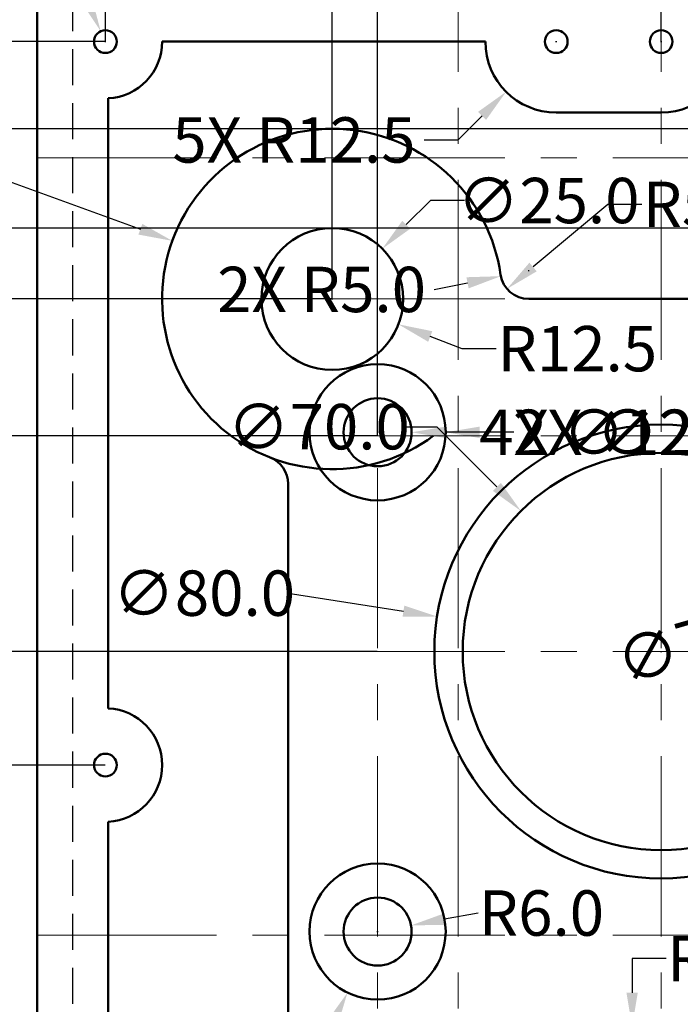
# Model space of a CAD drawing. Units: inches. Extents: x 11765 to 12471, y 10149 to 10793.
# Tile 4 of 8: x 11880 to 11996, y 10530 to 10704. Entities that reach past the tile are written whole.
import ezdxf

# ---------------------------------------------------------------- set-up
doc = ezdxf.new("R2010")
doc.units = ezdxf.units.IN
doc.header["$MEASUREMENT"] = 0
doc.linetypes.add('CENTER', pattern=[50.8, 31.75, -6.35, 6.35, -6.35])
doc.linetypes.add('HIDDEN', pattern=[9.525, 6.35, -3.175])
for name, color, linetype, lineweight in [('M-CNTR', 30, 'CENTER', 18), ('M-DIMS', 2, 'Continuous', 25), ('M-HIDN', 41, 'HIDDEN', 25), ('M-OUTL', 7, 'Continuous', 50)]:
    doc.layers.add(name, color=color, linetype=linetype, lineweight=lineweight)
doc.styles.get("Standard").update_dxf_attribs({"font": 'arial.ttf'})
doc.dimstyles.get("Standard").update_dxf_attribs({"dimtxt": 8, "dimasz": 6, "dimexe": 0.18, "dimexo": 0.0625, "dimgap": 0.09, "dimtad": 0, "dimtoh": 1, "dimdec": 1, "dimzin": 0, "dimdsep": 46, "dimtxsty": 'Standard', "dimcen": 0.09, "dimadec": 0, "dimazin": 0, "dimtfac": 1, "dimtdec": 1, "dimtofl": 0, "dimtmove": 0, "dimatfit": 3, "dimfxl": 1, "dimtolj": 1, "dimtzin": 0, "dimarcsym": 0})

# ---------------------------------------------------------------- blocks, each defined once
blk = doc.blocks.new('*D2')
at = {"layer": 'Defpoints', "color": 0, "transparency": 16777216}
for p in [(11894.91, 10776.05), (11992.91, 10712.15), (11894.91, 10699.65)]:
    blk.add_point(p, dxfattribs=at)
at = {"layer": 'M-DIMS', "color": 0, "lineweight": -2, "transparency": 16777216}
for p, q in [((11894.91, 10699.71), (11894.91, 10776.23)), ((11900.91, 10776.05), (11933.45, 10776.05)), ((11986.91, 10776.05), (11954.38, 10776.05)), ((11992.91, 10712.21), (11992.91, 10776.23))]:
    blk.add_line(p, q, dxfattribs=at)
at = {"layer": 'M-DIMS', "color": 0, "transparency": 16777216}
for points in [[(11900.91, 10777.05), (11900.91, 10775.05), (11894.91, 10776.05)], [(11986.91, 10777.05), (11986.91, 10775.05), (11992.91, 10776.05)]]:
    blk.add_solid(points, dxfattribs=at)
at = {"layer": 'M-DIMS', "color": 0, "transparency": 16777216, "insert": (11943.91, 10776.05), "char_height": 8, "attachment_point": 5}
blk.add_mtext('\\A1;98.0', dxfattribs=at)
blk = doc.blocks.new('*D3')
at = {"layer": 'Defpoints', "color": 0, "transparency": 16777216}
for p in [(11992.91, 10763.84), (11992.91, 10699.65), (11934.91, 10654.29)]:
    blk.add_point(p, dxfattribs=at)
at = {"layer": 'M-DIMS', "color": 0, "lineweight": -2, "transparency": 16777216}
for p, q in [((11934.91, 10654.35), (11934.91, 10764.02)), ((11940.91, 10763.84), (11953.45, 10763.84)), ((11986.91, 10763.84), (11974.38, 10763.84)), ((11992.91, 10699.71), (11992.91, 10764.02))]:
    blk.add_line(p, q, dxfattribs=at)
at = {"layer": 'M-DIMS', "color": 0, "transparency": 16777216}
for points in [[(11940.91, 10764.84), (11940.91, 10762.84), (11934.91, 10763.84)], [(11986.91, 10764.84), (11986.91, 10762.84), (11992.91, 10763.84)]]:
    blk.add_solid(points, dxfattribs=at)
at = {"layer": 'M-DIMS', "color": 0, "transparency": 16777216, "insert": (11963.91, 10763.84), "char_height": 8, "attachment_point": 5}
blk.add_mtext('\\A1;58.0', dxfattribs=at)
blk = doc.blocks.new('*D4')
at = {"layer": 'Defpoints', "color": 0, "transparency": 16777216}
for p in [(11992.91, 10750.16), (11992.91, 10699.65), (11942.91, 10630.15)]:
    blk.add_point(p, dxfattribs=at)
at = {"layer": 'M-DIMS', "color": 0, "lineweight": -2, "transparency": 16777216}
for p, q in [((11942.91, 10630.21), (11942.91, 10750.34)), ((11948.91, 10750.16), (11957.45, 10750.16)), ((11986.91, 10750.16), (11978.38, 10750.16)), ((11992.91, 10699.71), (11992.91, 10750.34))]:
    blk.add_line(p, q, dxfattribs=at)
at = {"layer": 'M-DIMS', "color": 0, "transparency": 16777216}
for points in [[(11948.91, 10751.16), (11948.91, 10749.16), (11942.91, 10750.16)], [(11986.91, 10751.16), (11986.91, 10749.16), (11992.91, 10750.16)]]:
    blk.add_solid(points, dxfattribs=at)
at = {"layer": 'M-DIMS', "color": 0, "transparency": 16777216, "insert": (11967.91, 10750.16), "char_height": 8, "attachment_point": 5}
blk.add_mtext('\\A1;50.0', dxfattribs=at)
blk = doc.blocks.new('*D5')
at = {"layer": 'Defpoints', "color": 0, "transparency": 16777216}
for p in [(11992.91, 10750.5), (11992.91, 10699.65), (12042.91, 10642.79)]:
    blk.add_point(p, dxfattribs=at)
at = {"layer": 'M-DIMS', "color": 0, "lineweight": -2, "transparency": 16777216}
for p, q in [((11992.91, 10699.71), (11992.91, 10750.68)), ((11998.91, 10750.5), (12007.45, 10750.5)), ((12036.91, 10750.5), (12028.38, 10750.5)), ((12042.91, 10642.86), (12042.91, 10750.68))]:
    blk.add_line(p, q, dxfattribs=at)
at = {"layer": 'M-DIMS', "color": 0, "transparency": 16777216}
for points in [[(11998.91, 10751.5), (11998.91, 10749.5), (11992.91, 10750.5)], [(12036.91, 10751.5), (12036.91, 10749.5), (12042.91, 10750.5)]]:
    blk.add_solid(points, dxfattribs=at)
at = {"layer": 'M-DIMS', "color": 0, "transparency": 16777216, "insert": (12017.91, 10750.5), "char_height": 8, "attachment_point": 5}
blk.add_mtext('\\A1;50.0', dxfattribs=at)
blk = doc.blocks.new('*D6')
at = {"layer": 'Defpoints', "color": 0, "transparency": 16777216}
for p in [(11882.91, 10712.15), (11769.87, 10237.15), (11917.55, 10237.15)]:
    blk.add_point(p, dxfattribs=at)
at = {"layer": 'M-DIMS', "color": 0, "lineweight": -2, "transparency": 16777216}
for p, q in [((11882.85, 10712.15), (11769.69, 10712.15)), ((11769.87, 10706.15), (11769.87, 10488.38)), ((11769.87, 10243.15), (11769.87, 10460.91)), ((11917.49, 10237.15), (11769.69, 10237.15))]:
    blk.add_line(p, q, dxfattribs=at)
at = {"layer": 'M-DIMS', "color": 0, "transparency": 16777216}
for points in [[(11768.87, 10706.15), (11770.87, 10706.15), (11769.87, 10712.15)], [(11768.87, 10243.15), (11770.87, 10243.15), (11769.87, 10237.15)]]:
    blk.add_solid(points, dxfattribs=at)
at = {"layer": 'M-DIMS', "color": 0, "transparency": 16777216, "insert": (11769.87, 10474.65), "char_height": 8, "attachment_point": 5, "rotation": 90}
blk.add_mtext('\\A1;475.0', dxfattribs=at)
blk = doc.blocks.new('*D14')
at = {"layer": 'Defpoints', "color": 0, "transparency": 16777216}
for p in [(12156.23, 10592.15), (12216.5, 10592.15), (11992.91, 10372.15)]:
    blk.add_point(p, dxfattribs=at)
at = {"layer": 'M-DIMS', "color": 0, "lineweight": -2, "transparency": 16777216}
for p, q in [((12156.3, 10592.15), (12216.68, 10592.15)), ((12216.5, 10586.15), (12216.5, 10495.79)), ((12216.5, 10378.15), (12216.5, 10468.5)), ((11992.97, 10372.15), (12216.68, 10372.15))]:
    blk.add_line(p, q, dxfattribs=at)
at = {"layer": 'M-DIMS', "color": 0, "transparency": 16777216}
for points in [[(12215.5, 10586.15), (12217.5, 10586.15), (12216.5, 10592.15)], [(12215.5, 10378.15), (12217.5, 10378.15), (12216.5, 10372.15)]]:
    blk.add_solid(points, dxfattribs=at)
at = {"layer": 'M-DIMS', "color": 0, "transparency": 16777216, "insert": (12216.5, 10482.15), "char_height": 8, "attachment_point": 5, "rotation": 90}
blk.add_mtext('\\A1;220.0', dxfattribs=at)
blk = doc.blocks.new('*D24')
at = {"layer": 'Defpoints', "color": 0, "transparency": 16777216}
for p in [(11794.92, 10712.15), (11882.91, 10712.15), (11882.91, 10592.15)]:
    blk.add_point(p, dxfattribs=at)
at = {"layer": 'M-DIMS', "color": 0, "lineweight": -2, "transparency": 16777216}
for p, q in [((11882.85, 10712.15), (11794.74, 10712.15)), ((11794.92, 10706.15), (11794.92, 10665.34)), ((11794.92, 10598.15), (11794.92, 10638.95)), ((11882.85, 10592.15), (11794.74, 10592.15))]:
    blk.add_line(p, q, dxfattribs=at)
at = {"layer": 'M-DIMS', "color": 0, "transparency": 16777216}
for points in [[(11793.92, 10706.15), (11795.92, 10706.15), (11794.92, 10712.15)], [(11793.92, 10598.15), (11795.92, 10598.15), (11794.92, 10592.15)]]:
    blk.add_solid(points, dxfattribs=at)
at = {"layer": 'M-DIMS', "color": 0, "transparency": 16777216, "insert": (11794.92, 10652.15), "char_height": 8, "attachment_point": 5, "rotation": 90}
blk.add_mtext('\\A1;120.0', dxfattribs=at)
blk = doc.blocks.new('*D25')
at = {"layer": 'Defpoints', "color": 0, "transparency": 16777216}
for p in [(11894.91, 10699.65), (11809.73, 10592.15), (11882.91, 10592.15)]:
    blk.add_point(p, dxfattribs=at)
at = {"layer": 'M-DIMS', "color": 0, "lineweight": -2, "transparency": 16777216}
for p, q in [((11894.85, 10699.65), (11809.55, 10699.65)), ((11809.73, 10693.65), (11809.73, 10659.14)), ((11809.73, 10598.15), (11809.73, 10632.65)), ((11882.85, 10592.15), (11809.55, 10592.15))]:
    blk.add_line(p, q, dxfattribs=at)
at = {"layer": 'M-DIMS', "color": 0, "transparency": 16777216}
for points in [[(11808.73, 10693.65), (11810.73, 10693.65), (11809.73, 10699.65)], [(11808.73, 10598.15), (11810.73, 10598.15), (11809.73, 10592.15)]]:
    blk.add_solid(points, dxfattribs=at)
at = {"layer": 'M-DIMS', "color": 0, "transparency": 16777216, "insert": (11809.73, 10645.9), "char_height": 8, "attachment_point": 5, "rotation": 90}
blk.add_mtext('\\A1;107.5', dxfattribs=at)
blk = doc.blocks.new('*D26')
at = {"layer": 'Defpoints', "color": 0, "transparency": 16777216}
for p in [(11934.91, 10654.29), (11823.92, 10592.15), (11882.91, 10592.15)]:
    blk.add_point(p, dxfattribs=at)
at = {"layer": 'M-DIMS', "color": 0, "lineweight": -2, "transparency": 16777216}
for p, q in [((11934.85, 10654.29), (11823.74, 10654.29)), ((11823.92, 10648.29), (11823.92, 10632.95)), ((11823.92, 10598.15), (11823.92, 10613.49)), ((11882.85, 10592.15), (11823.74, 10592.15))]:
    blk.add_line(p, q, dxfattribs=at)
at = {"layer": 'M-DIMS', "color": 0, "transparency": 16777216}
for points in [[(11822.92, 10648.29), (11824.92, 10648.29), (11823.92, 10654.29)], [(11822.92, 10598.15), (11824.92, 10598.15), (11823.92, 10592.15)]]:
    blk.add_solid(points, dxfattribs=at)
at = {"layer": 'M-DIMS', "color": 0, "transparency": 16777216, "insert": (11823.92, 10623.22), "char_height": 8, "attachment_point": 5, "rotation": 90}
blk.add_mtext('\\A1;62.1', dxfattribs=at)
blk = doc.blocks.new('*D27')
at = {"layer": 'Defpoints', "color": 0, "transparency": 16777216}
for p in [(11840.57, 10630.15), (11942.91, 10630.15), (11942.91, 10592.15)]:
    blk.add_point(p, dxfattribs=at)
at = {"layer": 'M-DIMS', "color": 0, "lineweight": -2, "transparency": 16777216}
for p, q in [((11942.85, 10630.15), (11840.39, 10630.15)), ((11840.57, 10624.15), (11840.57, 10621.61)), ((11840.57, 10598.15), (11840.57, 10600.68)), ((11942.85, 10592.15), (11840.39, 10592.15))]:
    blk.add_line(p, q, dxfattribs=at)
at = {"layer": 'M-DIMS', "color": 0, "transparency": 16777216}
for points in [[(11839.57, 10624.15), (11841.57, 10624.15), (11840.57, 10630.15)], [(11839.57, 10598.15), (11841.57, 10598.15), (11840.57, 10592.15)]]:
    blk.add_solid(points, dxfattribs=at)
at = {"layer": 'M-DIMS', "color": 0, "transparency": 16777216, "insert": (11840.57, 10611.15), "char_height": 8, "attachment_point": 5, "rotation": 90}
blk.add_mtext('\\A1;38.0', dxfattribs=at)
blk = doc.blocks.new('*D29')
at = {"layer": 'Defpoints', "color": 0, "transparency": 16777216}
for p in [(11794.06, 10592.15), (11889.16, 10592.15), (11894.91, 10322.15)]:
    blk.add_point(p, dxfattribs=at)
at = {"layer": 'M-DIMS', "color": 0, "lineweight": -2, "transparency": 16777216}
for p, q in [((11889.1, 10592.15), (11793.88, 10592.15)), ((11794.06, 10586.15), (11794.06, 10470.79)), ((11794.06, 10328.15), (11794.06, 10443.5)), ((11894.85, 10322.15), (11793.88, 10322.15))]:
    blk.add_line(p, q, dxfattribs=at)
at = {"layer": 'M-DIMS', "color": 0, "transparency": 16777216}
for points in [[(11793.06, 10586.15), (11795.06, 10586.15), (11794.06, 10592.15)], [(11793.06, 10328.15), (11795.06, 10328.15), (11794.06, 10322.15)]]:
    blk.add_solid(points, dxfattribs=at)
at = {"layer": 'M-DIMS', "color": 0, "transparency": 16777216, "insert": (11794.06, 10457.15), "char_height": 8, "attachment_point": 5, "rotation": 90}
blk.add_mtext('\\A1;270.0', dxfattribs=at)
blk = doc.blocks.new('*D30')
at = {"layer": 'Defpoints', "color": 0, "transparency": 16777216}
for p in [(11872.35, 10592.15), (11809.21, 10447.15), (11894.91, 10447.15)]:
    blk.add_point(p, dxfattribs=at)
at = {"layer": 'M-DIMS', "color": 0, "lineweight": -2, "transparency": 16777216}
for p, q in [((11872.29, 10592.15), (11809.03, 10592.15)), ((11809.21, 10586.15), (11809.21, 10532.84)), ((11809.21, 10453.15), (11809.21, 10506.45)), ((11894.85, 10447.15), (11809.03, 10447.15))]:
    blk.add_line(p, q, dxfattribs=at)
at = {"layer": 'M-DIMS', "color": 0, "transparency": 16777216}
for points in [[(11808.21, 10586.15), (11810.21, 10586.15), (11809.21, 10592.15)], [(11808.21, 10453.15), (11810.21, 10453.15), (11809.21, 10447.15)]]:
    blk.add_solid(points, dxfattribs=at)
at = {"layer": 'M-DIMS', "color": 0, "transparency": 16777216, "insert": (11809.21, 10519.65), "char_height": 8, "attachment_point": 5, "rotation": 90}
blk.add_mtext('\\A1;145.0', dxfattribs=at)
blk = doc.blocks.new('*D31')
at = {"layer": 'Defpoints', "color": 0, "transparency": 16777216}
for p in [(11895.41, 10592.15), (11874.92, 10572.15), (11894.91, 10572.15)]:
    blk.add_point(p, dxfattribs=at)
at = {"layer": 'M-DIMS', "color": 0, "lineweight": -2, "transparency": 16777216}
for p, q in [((11895.35, 10592.15), (11874.74, 10592.15)), ((11874.92, 10586.15), (11874.92, 10578.15)), ((11894.85, 10572.15), (11874.74, 10572.15)), ((11874.92, 10572.15), (11874.92, 10566.15)), ((11874.92, 10566.15), (11868.92, 10566.15))]:
    blk.add_line(p, q, dxfattribs=at)
at = {"layer": 'M-DIMS', "color": 0, "transparency": 16777216}
for points in [[(11873.92, 10586.15), (11875.92, 10586.15), (11874.92, 10592.15)], [(11873.92, 10578.15), (11875.92, 10578.15), (11874.92, 10572.15)]]:
    blk.add_solid(points, dxfattribs=at)
at = {"layer": 'M-DIMS', "color": 0, "transparency": 16777216, "insert": (11858.38, 10566.15), "char_height": 8, "attachment_point": 5}
blk.add_mtext('\\A1;20.0', dxfattribs=at)
blk = doc.blocks.new('*D33')
at = {"layer": 'Defpoints', "color": 0, "transparency": 16777216}
for p in [(11992.91, 10699.65), (11999.97, 10689.33)]:
    blk.add_point(p, dxfattribs=at)
at = {"layer": 'M-DIMS', "color": 0, "lineweight": -2, "transparency": 16777216}
for p, q in [((11992.82, 10699.65), (11993, 10699.65)), ((11992.91, 10699.56), (11992.91, 10699.74)), ((12006.75, 10679.43), (12003.36, 10684.38)), ((12012.75, 10679.43), (12006.75, 10679.43))]:
    blk.add_line(p, q, dxfattribs=at)
at = {"layer": 'M-DIMS', "color": 0, "transparency": 16777216}
blk.add_solid([(12004.19, 10684.95), (12002.54, 10683.82), (11999.97, 10689.33)], dxfattribs=at)
at = {"layer": 'M-DIMS', "color": 0, "transparency": 16777216, "insert": (12027.09, 10679.43), "char_height": 8, "attachment_point": 5}
blk.add_mtext('\\A1;R12.5', dxfattribs=at)
blk = doc.blocks.new('*D34')
at = {"layer": 'Defpoints', "color": 0, "transparency": 16777216}
for p in [(11969.55, 10659.29), (11965.72, 10656.07)]:
    blk.add_point(p, dxfattribs=at)
at = {"layer": 'M-DIMS', "color": 0, "lineweight": -2, "transparency": 16777216}
for p, q in [((11983.49, 10670.97), (11970.32, 10659.93)), ((11989.49, 10670.97), (11983.49, 10670.97))]:
    blk.add_line(p, q, dxfattribs=at)
at = {"layer": 'M-DIMS', "color": 0, "transparency": 16777216}
blk.add_solid([(11969.68, 10660.69), (11970.96, 10659.16), (11965.72, 10656.07)], dxfattribs=at)
at = {"layer": 'M-DIMS', "color": 0, "transparency": 16777216, "insert": (12000.68, 10670.97), "char_height": 8, "attachment_point": 5}
blk.add_mtext('\\A1;R5.0', dxfattribs=at)
blk = doc.blocks.new('*D35')
at = {"layer": 'Defpoints', "color": 0, "transparency": 16777216}
for p in [(11906.72, 10664.53), (11934.91, 10654.29)]:
    blk.add_point(p, dxfattribs=at)
at = {"layer": 'M-DIMS', "color": 0, "lineweight": -2, "transparency": 16777216}
for p, q in [((11862.11, 10678.56), (11868.11, 10678.56)), ((11868.11, 10678.56), (11901.08, 10666.58)), ((11934.82, 10654.29), (11935, 10654.29)), ((11934.91, 10654.2), (11934.91, 10654.38))]:
    blk.add_line(p, q, dxfattribs=at)
at = {"layer": 'M-DIMS', "color": 0, "transparency": 16777216}
blk.add_solid([(11901.42, 10667.52), (11900.74, 10665.64), (11906.72, 10664.53)], dxfattribs=at)
at = {"layer": 'M-DIMS', "color": 0, "transparency": 16777216, "insert": (11847.81, 10678.56), "char_height": 8, "attachment_point": 5}
blk.add_mtext('\\A1;R30.0', dxfattribs=at)
blk = doc.blocks.new('*D36')
at = {"layer": 'Defpoints', "color": 0, "transparency": 16777216}
for p in [(11934.91, 10654.29), (11946.59, 10649.82)]:
    blk.add_point(p, dxfattribs=at)
at = {"layer": 'M-DIMS', "color": 0, "lineweight": -2, "transparency": 16777216}
for p, q in [((11934.82, 10654.29), (11935, 10654.29)), ((11934.91, 10654.2), (11934.91, 10654.38)), ((11957.79, 10645.53), (11952.19, 10647.67)), ((11963.79, 10645.53), (11957.79, 10645.53))]:
    blk.add_line(p, q, dxfattribs=at)
at = {"layer": 'M-DIMS', "color": 0, "transparency": 16777216}
blk.add_solid([(11952.55, 10648.61), (11951.83, 10646.74), (11946.59, 10649.82)], dxfattribs=at)
at = {"layer": 'M-DIMS', "color": 0, "transparency": 16777216, "insert": (11978.13, 10645.53), "char_height": 8, "attachment_point": 5}
blk.add_mtext('\\A1;R12.5', dxfattribs=at)
blk = doc.blocks.new('*D39')
at = {"layer": 'Defpoints', "color": 0, "transparency": 16777216}
for p in [(11942.91, 10542.79), (11937.6, 10532.03)]:
    blk.add_point(p, dxfattribs=at)
at = {"layer": 'M-DIMS', "color": 0, "lineweight": -2, "transparency": 16777216}
for p, q in [((11942.82, 10542.79), (11943, 10542.79)), ((11942.91, 10542.7), (11942.91, 10542.88)), ((11932.3, 10521.27), (11934.95, 10526.65)), ((11926.3, 10521.27), (11932.3, 10521.27))]:
    blk.add_line(p, q, dxfattribs=at)
at = {"layer": 'M-DIMS', "color": 0, "transparency": 16777216}
blk.add_solid([(11934.05, 10527.09), (11935.85, 10526.21), (11937.6, 10532.03)], dxfattribs=at)
at = {"layer": 'M-DIMS', "color": 0, "transparency": 16777216, "insert": (11912, 10521.27), "char_height": 8, "attachment_point": 5}
blk.add_mtext('\\A1;R12.0', dxfattribs=at)
blk = doc.blocks.new('*D40')
at = {"layer": 'Defpoints', "color": 0, "transparency": 16777216}
for p in [(11942.91, 10542.79), (11948.81, 10543.88)]:
    blk.add_point(p, dxfattribs=at)
at = {"layer": 'M-DIMS', "color": 0, "lineweight": -2, "transparency": 16777216}
for p, q in [((11960.61, 10546.06), (11954.71, 10544.97)), ((11942.82, 10542.79), (11943, 10542.79)), ((11942.91, 10542.7), (11942.91, 10542.88))]:
    blk.add_line(p, q, dxfattribs=at)
at = {"layer": 'M-DIMS', "color": 0, "transparency": 16777216}
blk.add_solid([(11954.53, 10545.95), (11954.89, 10543.98), (11948.81, 10543.88)], dxfattribs=at)
at = {"layer": 'M-DIMS', "color": 0, "transparency": 16777216, "insert": (11971.8, 10546.06), "char_height": 8, "attachment_point": 5}
blk.add_mtext('\\A1;R6.0', dxfattribs=at)
blk = doc.blocks.new('*D41')
at = {"layer": 'Defpoints', "color": 0, "transparency": 16777216}
for p in [(11987.78, 10526.02), (11987.78, 10521.02)]:
    blk.add_point(p, dxfattribs=at)
at = {"layer": 'M-DIMS', "color": 0, "lineweight": -2, "transparency": 16777216}
for p, q in [((11993.78, 10538.02), (11987.78, 10538.02)), ((11987.78, 10538.02), (11987.78, 10532.02)), ((11987.69, 10521.02), (11987.87, 10521.02)), ((11987.78, 10520.93), (11987.78, 10521.11))]:
    blk.add_line(p, q, dxfattribs=at)
at = {"layer": 'M-DIMS', "color": 0, "transparency": 16777216}
blk.add_solid([(11986.78, 10532.02), (11988.78, 10532.02), (11987.78, 10526.02)], dxfattribs=at)
at = {"layer": 'M-DIMS', "color": 0, "transparency": 16777216, "insert": (12004.97, 10538.02), "char_height": 8, "attachment_point": 5}
blk.add_mtext('\\A1;R5.0', dxfattribs=at)
blk = doc.blocks.new('*D42')
at = {"layer": 'Defpoints', "color": 0, "transparency": 16777216}
for p in [(12026.53, 10601.87), (11959.29, 10582.42)]:
    blk.add_point(p, dxfattribs=at)
at = {"layer": 'M-DIMS', "color": 0, "lineweight": -2, "transparency": 16777216}
blk.add_line((12015.01, 10598.54), (12020.77, 10600.2), dxfattribs=at)
at = {"layer": 'M-DIMS', "color": 0, "transparency": 16777216}
blk.add_solid([(12020.49, 10601.16), (12021.05, 10599.24), (12026.53, 10601.87)], dxfattribs=at)
at = {"layer": 'M-DIMS', "color": 0, "transparency": 16777216, "insert": (12000.77, 10594.42), "char_height": 8, "attachment_point": 5, "rotation": 16.1306}
blk.add_mtext('\\A1;∅70.0', dxfattribs=at)
blk = doc.blocks.new('*D43')
at = {"layer": 'Defpoints', "color": 0, "transparency": 16777216}
for p in [(11953.39, 10598.33), (12032.43, 10585.96)]:
    blk.add_point(p, dxfattribs=at)
at = {"layer": 'M-DIMS', "color": 0, "lineweight": -2, "transparency": 16777216}
for p, q in [((11927.12, 10602.44), (11947.47, 10599.26)), ((11992.82, 10592.15), (11993, 10592.15)), ((11992.91, 10592.06), (11992.91, 10592.24))]:
    blk.add_line(p, q, dxfattribs=at)
at = {"layer": 'M-DIMS', "color": 0, "transparency": 16777216}
blk.add_solid([(11947.62, 10600.25), (11947.31, 10598.27), (11953.39, 10598.33)], dxfattribs=at)
at = {"layer": 'M-DIMS', "color": 0, "transparency": 16777216, "insert": (11912.3, 10602.44), "char_height": 8, "attachment_point": 5}
blk.add_mtext('\\A1;∅80.0', dxfattribs=at)
blk = doc.blocks.new('*D62')
at = {"layer": 'Defpoints', "color": 0, "transparency": 16777216}
for p in [(12379.9, 10706.15), (11848.16, 10684.29), (12385.4, 10684.29)]:
    blk.add_point(p, dxfattribs=at)
at = {"layer": 'M-DIMS', "color": 0, "lineweight": -2, "transparency": 16777216}
for p, q in [((12379.83, 10706.15), (11847.98, 10706.15)), ((11848.16, 10700.15), (11848.16, 10690.29)), ((12385.33, 10684.29), (11847.98, 10684.29)), ((11848.16, 10684.29), (11848.16, 10678.29)), ((11848.16, 10678.29), (11842.16, 10678.29))]:
    blk.add_line(p, q, dxfattribs=at)
at = {"layer": 'M-DIMS', "color": 0, "transparency": 16777216}
for points in [[(11847.16, 10700.15), (11849.16, 10700.15), (11848.16, 10706.15)], [(11847.16, 10690.29), (11849.16, 10690.29), (11848.16, 10684.29)]]:
    blk.add_solid(points, dxfattribs=at)
at = {"layer": 'M-DIMS', "color": 0, "transparency": 16777216, "insert": (11828.51, 10678.29), "char_height": 8, "attachment_point": 5}
blk.add_mtext('\\A1;21.86', dxfattribs=at)
blk = doc.blocks.new('*D63')
at = {"layer": 'Defpoints', "color": 0, "transparency": 16777216}
for p in [(12385.4, 10684.29), (11848.16, 10666.79), (12385.4, 10666.79)]:
    blk.add_point(p, dxfattribs=at)
at = {"layer": 'M-DIMS', "color": 0, "lineweight": -2, "transparency": 16777216}
for p, q in [((12385.33, 10684.29), (11847.98, 10684.29)), ((11848.16, 10678.29), (11848.16, 10672.79)), ((12385.33, 10666.79), (11847.98, 10666.79)), ((11848.16, 10666.79), (11848.16, 10660.79)), ((11848.16, 10660.79), (11842.16, 10660.79))]:
    blk.add_line(p, q, dxfattribs=at)
at = {"layer": 'M-DIMS', "color": 0, "transparency": 16777216}
for points in [[(11847.16, 10678.29), (11849.16, 10678.29), (11848.16, 10684.29)], [(11847.16, 10672.79), (11849.16, 10672.79), (11848.16, 10666.79)]]:
    blk.add_solid(points, dxfattribs=at)
at = {"layer": 'M-DIMS', "color": 0, "transparency": 16777216, "insert": (11832.03, 10660.79), "char_height": 8, "attachment_point": 5}
blk.add_mtext('\\A1;17.5', dxfattribs=at)
blk = doc.blocks.new('*D68')
at = {"layer": 'Defpoints', "color": 0, "transparency": 16777216}
for p in [(11964.61, 10620.41), (12021.22, 10563.88)]:
    blk.add_point(p, dxfattribs=at)
at = {"layer": 'M-DIMS', "color": 0, "lineweight": -2, "transparency": 16777216}
for p, q in [((11992.82, 10592.15), (11993, 10592.15)), ((11992.91, 10592.06), (11992.91, 10592.24)), ((12038.2, 10546.92), (12025.46, 10559.64)), ((12044.2, 10546.92), (12038.2, 10546.92))]:
    blk.add_line(p, q, dxfattribs=at)
at = {"layer": 'M-DIMS', "color": 0, "transparency": 16777216}
blk.add_solid([(12026.17, 10560.35), (12024.76, 10558.94), (12021.22, 10563.88)], dxfattribs=at)
at = {"layer": 'M-DIMS', "color": 0, "transparency": 16777216, "insert": (12059.02, 10546.92), "char_height": 8, "attachment_point": 5}
blk.add_mtext('\\A1;∅80.0', dxfattribs=at)
blk = doc.blocks.new('*D69')
at = {"layer": 'Defpoints', "color": 0, "transparency": 16777216}
for p in [(11968.18, 10616.92), (12017.64, 10567.38)]:
    blk.add_point(p, dxfattribs=at)
at = {"layer": 'M-DIMS', "color": 0, "lineweight": -2, "transparency": 16777216}
for p, q in [((11947.35, 10631.78), (11953.35, 10631.78)), ((11953.35, 10631.78), (11963.95, 10621.16)), ((11992.82, 10592.15), (11993, 10592.15)), ((11992.91, 10592.06), (11992.91, 10592.24))]:
    blk.add_line(p, q, dxfattribs=at)
at = {"layer": 'M-DIMS', "color": 0, "transparency": 16777216}
blk.add_solid([(11964.65, 10621.87), (11963.24, 10620.46), (11968.18, 10616.92)], dxfattribs=at)
at = {"layer": 'M-DIMS', "color": 0, "transparency": 16777216, "insert": (11932.53, 10631.78), "char_height": 8, "attachment_point": 5}
blk.add_mtext('\\A1;∅70.0', dxfattribs=at)
blk = doc.blocks.new('*D76')
at = {"layer": 'Defpoints', "color": 0, "transparency": 16777216}
for p in [(11943.74, 10663.14), (11926.09, 10645.43)]:
    blk.add_point(p, dxfattribs=at)
at = {"layer": 'M-DIMS', "color": 0, "lineweight": -2, "transparency": 16777216}
for p, q in [((11952.21, 10671.64), (11947.97, 10667.39)), ((11958.21, 10671.64), (11952.21, 10671.64)), ((11934.82, 10654.29), (11935, 10654.29)), ((11934.91, 10654.2), (11934.91, 10654.38))]:
    blk.add_line(p, q, dxfattribs=at)
at = {"layer": 'M-DIMS', "color": 0, "transparency": 16777216}
blk.add_solid([(11947.27, 10668.09), (11948.68, 10666.68), (11943.74, 10663.14)], dxfattribs=at)
at = {"layer": 'M-DIMS', "color": 0, "transparency": 16777216, "insert": (11973.03, 10671.64), "char_height": 8, "attachment_point": 5}
blk.add_mtext('\\A1;∅25.0', dxfattribs=at)
blk = doc.blocks.new('*D77')
at = {"layer": 'Defpoints', "color": 0, "transparency": 16777216}
for p in [(11974.41, 10699.65), (11965.57, 10690.81)]:
    blk.add_point(p, dxfattribs=at)
at = {"layer": 'M-DIMS', "color": 0, "lineweight": -2, "transparency": 16777216}
for p, q in [((11974.32, 10699.65), (11974.5, 10699.65)), ((11974.41, 10699.56), (11974.41, 10699.74)), ((11957.09, 10682.32), (11961.33, 10686.56)), ((11951.09, 10682.32), (11957.09, 10682.32))]:
    blk.add_line(p, q, dxfattribs=at)
at = {"layer": 'M-DIMS', "color": 0, "transparency": 16777216}
blk.add_solid([(11960.62, 10687.27), (11962.04, 10685.86), (11965.57, 10690.81)], dxfattribs=at)
at = {"layer": 'M-DIMS', "color": 0, "transparency": 16777216, "insert": (11928.15, 10682.32), "char_height": 8, "attachment_point": 5}
blk.add_mtext('\\A1;5X R12.5', dxfattribs=at)
blk = doc.blocks.new('*D78')
at = {"layer": 'Defpoints', "color": 0, "transparency": 16777216}
for p in [(11930.91, 10630.79), (11954.91, 10630.79)]:
    blk.add_point(p, dxfattribs=at)
at = {"layer": 'M-DIMS', "color": 0, "lineweight": -2, "transparency": 16777216}
for p, q in [((11942.82, 10630.79), (11943, 10630.79)), ((11942.91, 10630.7), (11942.91, 10630.88)), ((11966.91, 10630.79), (11960.91, 10630.79))]:
    blk.add_line(p, q, dxfattribs=at)
at = {"layer": 'M-DIMS', "color": 0, "transparency": 16777216}
blk.add_solid([(11960.91, 10631.79), (11960.91, 10629.79), (11954.91, 10630.79)], dxfattribs=at)
at = {"layer": 'M-DIMS', "color": 0, "transparency": 16777216, "insert": (11990.18, 10630.79), "char_height": 8, "attachment_point": 5}
blk.add_mtext('\\A1;2X ∅24.0', dxfattribs=at)
blk = doc.blocks.new('*D81')
at = {"layer": 'Defpoints', "color": 0, "transparency": 16777216}
for p in [(11936.91, 10630.79), (11948.91, 10630.79)]:
    blk.add_point(p, dxfattribs=at)
at = {"layer": 'M-DIMS', "color": 0, "lineweight": -2, "transparency": 16777216}
for p, q in [((11942.82, 10630.79), (11943, 10630.79)), ((11942.91, 10630.7), (11942.91, 10630.88)), ((11960.91, 10630.79), (11954.91, 10630.79))]:
    blk.add_line(p, q, dxfattribs=at)
at = {"layer": 'M-DIMS', "color": 0, "transparency": 16777216}
blk.add_solid([(11954.91, 10631.79), (11954.91, 10629.79), (11948.91, 10630.79)], dxfattribs=at)
at = {"layer": 'M-DIMS', "color": 0, "transparency": 16777216, "insert": (11984.27, 10630.79), "char_height": 8, "attachment_point": 5}
blk.add_mtext('\\A1;4X ∅12.0', dxfattribs=at)
blk = doc.blocks.new('*D82')
at = {"layer": 'Defpoints', "color": 0, "transparency": 16777216}
for p in [(11969.55, 10659.29), (11964.65, 10658.31)]:
    blk.add_point(p, dxfattribs=at)
at = {"layer": 'M-DIMS', "color": 0, "lineweight": -2, "transparency": 16777216}
for p, q in [((11969.46, 10659.29), (11969.64, 10659.29)), ((11969.55, 10659.2), (11969.55, 10659.38)), ((11952.88, 10655.97), (11958.76, 10657.14))]:
    blk.add_line(p, q, dxfattribs=at)
at = {"layer": 'M-DIMS', "color": 0, "transparency": 16777216}
blk.add_solid([(11958.57, 10658.12), (11958.96, 10656.16), (11964.65, 10658.31)], dxfattribs=at)
at = {"layer": 'M-DIMS', "color": 0, "transparency": 16777216, "insert": (11933.03, 10655.97), "char_height": 8, "attachment_point": 5}
blk.add_mtext('\\A1;2X R5.0', dxfattribs=at)
blk = doc.blocks.new('*D83')
at = {"layer": 'Defpoints', "color": 0, "transparency": 16777216}
for p in [(11894.09, 10701.47), (11895.73, 10697.82)]:
    blk.add_point(p, dxfattribs=at)
at = {"layer": 'M-DIMS', "color": 0, "lineweight": -2, "transparency": 16777216}
for p, q in [((11883.16, 10712.41), (11889.16, 10712.41)), ((11889.16, 10712.41), (11891.62, 10706.94)), ((11894.82, 10699.65), (11895, 10699.65)), ((11894.91, 10699.56), (11894.91, 10699.74))]:
    blk.add_line(p, q, dxfattribs=at)
at = {"layer": 'M-DIMS', "color": 0, "transparency": 16777216}
blk.add_solid([(11892.53, 10707.35), (11890.71, 10706.53), (11894.09, 10701.47)], dxfattribs=at)
at = {"layer": 'M-DIMS', "color": 0, "transparency": 16777216, "insert": (11860.33, 10712.41), "char_height": 8, "attachment_point": 5}
blk.add_mtext('\\A1;13X ∅4.0', dxfattribs=at)

msp = doc.modelspace()

# ---------------------------------------------------------------- linework, layer by layer
at = {"layer": 'M-CNTR'}
for p, q in [((11942.912, 10237.146), (11942.912, 10712.146)), ((11957.122, 10237.146), (11957.122, 10712.146)), ((11992.912, 10237.146), (11992.912, 10712.146)), ((12066.912, 10679.146), (11882.912, 10679.146)), ((12066.912, 10654.286), (11882.912, 10654.286)), ((12066.912, 10630.146), (11882.912, 10630.146)), ((12066.912, 10592.146), (11882.912, 10592.146)), ((12066.912, 10542.146), (11882.912, 10542.146))]:
    msp.add_line(p, q, dxfattribs=at)
at = {"layer": 'M-HIDN'}
msp.add_lwpolyline([(12060.662, 10705.896), (12060.662, 10515.896), (12096.662, 10515.896), (12096.662, 10263.352), (12062.096, 10243.396), (11923.728, 10243.396), (11889.162, 10263.352), (11889.162, 10705.896)], close=True, dxfattribs=at)
at = {"layer": 'M-OUTL'}
for p, q in [((11882.912, 10712.146), (11882.912, 10257.146)), ((11961.912, 10699.646), (11904.912, 10699.646)), ((11895.412, 10689.658), (11895.412, 10582.133)), ((11992.912, 10687.146), (11974.412, 10687.146)), ((11969.553, 10654.286), (12052.912, 10654.286)), ((11927.122, 10504.146), (11927.122, 10621.706)), ((11895.412, 10562.158), (11895.412, 10457.133))]:
    msp.add_line(p, q, dxfattribs=at)
for centre, radius in [((11894.912, 10699.646), 2), ((11974.412, 10699.646), 2), ((11992.912, 10699.646), 2), ((11934.912, 10654.286), 12.5), ((11942.912, 10630.793), 12), ((11942.912, 10630.793), 6), ((11992.912, 10592.146), 40), ((11992.912, 10592.146), 35), ((11894.912, 10572.146), 2), ((11942.912, 10542.793), 12), ((11942.912, 10542.793), 6)]:
    msp.add_circle(centre, radius, dxfattribs=at)
for centre, radius, start, end in [((11894.912, 10699.646), 10, 272.86598, 0), ((11974.412, 10699.646), 12.5, 180, 270), ((11992.912, 10699.646), 12.5, 270, 0), ((11934.912, 10654.286), 30, 8.21321, 306.42192), ((11969.553, 10659.286), 5, 188.21321, 270), ((11922.122, 10621.706), 5, 0, 68.56604), ((11894.912, 10572.146), 10, 272.86598, 87.13402)]:
    msp.add_arc(centre, radius, start, end, dxfattribs=at)

# ---------------------------------------------------------------- dimensions: what is measured, and where the dimension line sits
at = {"layer": 'M-DIMS'}
for base, p1, p2, picture, middle in [((11894.912, 10776.05), (11992.912, 10712.146), (11894.912, 10699.646), '*D2', (11943.912, 10776.05)), ((11992.912, 10763.836), (11934.912, 10654.286), (11992.912, 10699.646), '*D3', (11963.912, 10763.836)), ((11992.912, 10750.16), (11942.912, 10630.146), (11992.912, 10699.646), '*D4', (11967.912, 10750.16)), ((11992.912, 10750.499), (12042.912, 10642.793), (11992.912, 10699.646), '*D5', (12017.912, 10750.499))]:
    dim = msp.add_linear_dim(base=base, p1=p1, p2=p2, dimstyle='Standard', override={"dimclrd": 0, "dimclre": 0, "dimclrt": 0}, dxfattribs=at)
    dim.commit()
    dim.dimension.update_dxf_attribs({"geometry": picture, "text_midpoint": middle})
for p1, p2, text, picture, middle in [((11895.734, 10697.822), (11894.09, 10701.469), '13X <>', '*D83', (11860.332, 10712.407)), ((11930.912, 10630.793), (11954.912, 10630.793), '2X <>', '*D78', (11966.912, 10630.793)), ((11936.912, 10630.793), (11948.912, 10630.793), '4X <>', '*D81', (11960.912, 10630.793))]:
    dim = msp.add_diameter_dim_2p(p1=p1, p2=p2, text=text, dimstyle='Standard', override={"dimdec": 1, "dimlfac": 1, "dimrnd": 0, "dimzin": 0, "dimdsep": 46, "dimlunit": 2}, dxfattribs=at)
    dim.commit()
    dim.dimension.update_dxf_attribs({"geometry": picture, "text_midpoint": middle, "dimtype": 163})
for base, p1, p2, override, picture, middle in [((11769.869, 10237.146), (11882.912, 10712.146), (11917.553, 10237.146), {"dimclrd": 0, "dimclre": 0, "dimclrt": 0}, '*D6', (11769.869, 10474.646)), ((11794.917, 10712.146), (11882.912, 10592.146), (11882.912, 10712.146), {"dimclrd": 0, "dimclre": 0, "dimclrt": 0}, '*D24', (11794.917, 10652.146)), ((11848.162, 10684.286), (12379.896, 10706.146), (12385.396, 10684.286), {"dimdec": 2, "dimlfac": 1, "dimrnd": 0, "dimzin": 0, "dimdsep": 46, "dimlunit": 2}, '*D62', (11828.509, 10678.286)), ((11809.731, 10592.146), (11894.912, 10699.646), (11882.912, 10592.146), {"dimclrd": 0, "dimclre": 0, "dimclrt": 0}, '*D25', (11809.731, 10645.896)), ((11848.162, 10666.786), (12385.396, 10684.286), (12385.396, 10666.786), {"dimdec": 1, "dimlfac": 1, "dimrnd": 0, "dimzin": 0, "dimdsep": 46, "dimlunit": 2}, '*D63', (11832.028, 10660.786)), ((11823.918, 10592.146), (11934.912, 10654.286), (11882.912, 10592.146), {"dimclrd": 0, "dimclre": 0, "dimclrt": 0}, '*D26', (11823.918, 10623.216)), ((11840.567, 10630.146), (11942.912, 10592.146), (11942.912, 10630.146), {"dimclrd": 0, "dimclre": 0, "dimclrt": 0}, '*D27', (11840.567, 10611.146)), ((11794.063, 10592.146), (11894.912, 10322.146), (11889.162, 10592.146), {"dimclrd": 0, "dimclre": 0, "dimclrt": 0}, '*D29', (11794.063, 10457.146)), ((11809.207, 10447.146), (11872.348, 10592.146), (11894.912, 10447.146), {"dimclrd": 0, "dimclre": 0, "dimclrt": 0}, '*D30', (11809.207, 10519.646)), ((11874.915, 10572.146), (11895.412, 10592.146), (11894.912, 10572.146), {"dimclrd": 0, "dimclre": 0, "dimclrt": 0}, '*D31', (11858.381, 10566.146)), ((12216.505, 10592.146), (11992.912, 10372.146), (12156.234, 10592.146), {"dimclrd": 0, "dimclre": 0, "dimclrt": 0}, '*D14', (12216.505, 10482.146))]:
    dim = msp.add_linear_dim(base=base, p1=p1, p2=p2, angle=90, dimstyle='Standard', override=override, dxfattribs=at)
    dim.commit()
    dim.dimension.update_dxf_attribs({"geometry": picture, "text_midpoint": middle})
for center, mpoint, text, picture, middle in [((11974.412, 10699.646), (11965.573, 10690.807), '5X <>', '*D77', (11928.154, 10682.322)), ((11969.553, 10659.286), (11964.649, 10658.311), '2X <>', '*D82', (11933.029, 10655.972))]:
    dim = msp.add_radius_dim(center=center, mpoint=mpoint, text=text, dimstyle='Standard', override={"dimdec": 1, "dimlfac": 1, "dimrnd": 0, "dimzin": 0, "dimdsep": 46, "dimlunit": 2}, dxfattribs=at)
    dim.commit()
    dim.dimension.update_dxf_attribs({"geometry": picture, "text_midpoint": middle})
for center, mpoint, picture, middle in [((11992.912, 10699.646), (11999.974, 10689.332), '*D33', (12027.093, 10679.431)), ((11934.912, 10654.286), (11946.586, 10649.817), '*D36', (11978.131, 10645.528)), ((11942.912, 10542.793), (11948.813, 10543.88), '*D40', (11971.801, 10546.056)), ((11942.912, 10542.793), (11937.604, 10532.031), '*D39', (11912.001, 10521.268)), ((11987.783, 10521.025), (11987.783, 10526.025), '*D41', (12004.97, 10538.025))]:
    dim = msp.add_radius_dim(center=center, mpoint=mpoint, dimstyle='Standard', override={"dimclrd": 0, "dimclre": 0, "dimclrt": 0}, dxfattribs=at)
    dim.commit()
    dim.dimension.update_dxf_attribs({"geometry": picture, "text_midpoint": middle})
for center, mpoint, picture, middle in [((11934.912, 10654.286), (11906.716, 10664.533), '*D35', (11847.813, 10678.564)), ((11969.553, 10659.286), (11965.721, 10656.074), '*D34', (12000.68, 10670.966))]:
    dim = msp.add_radius_dim(center=center, mpoint=mpoint, dimstyle='Standard', override={"dimclrd": 0, "dimclre": 0, "dimclrt": 0}, dxfattribs=at)
    dim.commit()
    dim.dimension.update_dxf_attribs({"geometry": picture, "text_midpoint": middle, "dimtype": 164})
for p1, p2, override, picture, middle in [((11926.086, 10645.433), (11943.738, 10663.138), {"dimdec": 1, "dimlfac": 1, "dimrnd": 0, "dimzin": 0, "dimdsep": 46, "dimlunit": 2}, '*D76', (11973.029, 10671.636)), ((12017.639, 10567.376), (11968.185, 10616.916), {"dimdec": 1, "dimlfac": 1, "dimrnd": 0, "dimzin": 0, "dimdsep": 46, "dimlunit": 2}, '*D69', (11932.529, 10631.777)), ((11964.607, 10620.409), (12021.217, 10563.883), {"dimdec": 1, "dimlfac": 1, "dimrnd": 0, "dimzin": 0, "dimdsep": 46, "dimlunit": 2}, '*D68', (12059.019, 10546.925)), ((12032.431, 10585.96), (11953.393, 10598.331), {"dimclrd": 0, "dimclre": 0, "dimclrt": 0}, '*D43', (11927.122, 10602.444)), ((11959.29, 10582.422), (12026.534, 10601.87), {"dimclrd": 0, "dimclre": 0, "dimclrt": 0}, '*D42', (12000.771, 10594.419))]:
    dim = msp.add_diameter_dim_2p(p1=p1, p2=p2, dimstyle='Standard', override=override, dxfattribs=at)
    dim.commit()
    dim.dimension.update_dxf_attribs({"geometry": picture, "text_midpoint": middle, "dimtype": 163})

doc.saveas('drawing.dxf')
